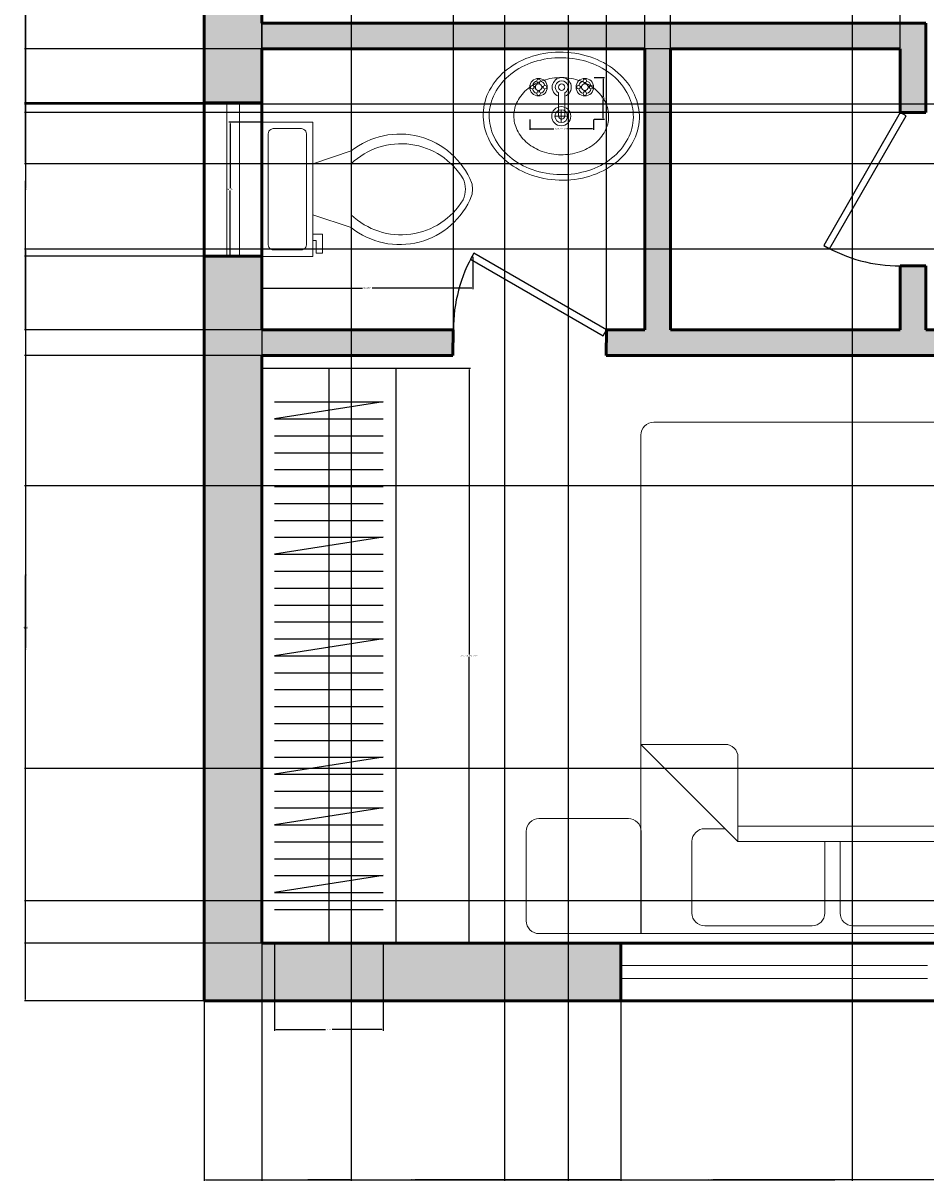
# Model space of a CAD drawing. Units: inches. Extents: x 1869 to 2483, y 2084 to 2479.
# Tile 1 of 7: x 1869 to 2010, y 2084 to 2265. Entities that reach past the tile are written whole.
import ezdxf

# ---------------------------------------------------------------- set-up
doc = ezdxf.new("R2010")
doc.units = ezdxf.units.IN
for name, color, linetype, lineweight in [('A-ANNO-DIMS', 2, 'Continuous', 18), ('A-DOOR', 3, 'Continuous', 25), ('A-FLOR-CASE', 9, 'Continuous', 25), ('A-FLOR-FIXT', 9, 'Continuous', 18), ('A-FURN', 8, 'Continuous', 18), ('A-GLAZ', 4, 'Continuous', 18), ('A-WALL', 7, 'Continuous', 50)]:
    doc.layers.add(name, color=color, linetype=linetype, lineweight=lineweight)
doc.layers.add('A-WALL-PATT', color=18, linetype='Continuous', lineweight=13, true_color=0x000000)
doc.styles.get("Standard").update_dxf_attribs({"font": 'arial.ttf'})
doc.dimstyles.get("Standard").update_dxf_attribs({"dimtxt": 0.18, "dimasz": 0.18, "dimexe": 0.18, "dimexo": 0.0625, "dimgap": 0.09, "dimtad": 0, "dimtih": 1, "dimtoh": 1, "dimdec": 4, "dimzin": 0, "dimdsep": 46, "dimtxsty": 'Standard', "dimcen": 0.09, "dimadec": 0, "dimazin": 0, "dimtfac": 1, "dimtdec": 4, "dimtofl": 0, "dimtmove": 0, "dimatfit": 3, "dimfxl": 1, "dimtolj": 1, "dimtzin": 0, "dimarcsym": 0})

# ---------------------------------------------------------------- blocks, each defined once
blk = doc.blocks.new('Sink - Oval top')
for p, q in [((-1, 0), (1, 0)), ((0, 1), (0, -1))]:
    blk.add_line(p, q)
for points in [[(-12.23, 0.39, 0.117634), (-11.46, -3.36, 0.104469), (-8.88, -6.8, 0.090016), (-5.08, -9.07, 0.08192), (-0.32, -10.02, 0.08192), (4.49, -9.38, 0.090016), (8.42, -7.36, 0.104469), (11.22, -4.09, 0.117634), (12.23, -0.39, 0.117634), (11.46, 3.36, 0.104469), (8.88, 6.8, 0.090016), (5.08, 9.07, 0.08192), (0.32, 10.02, 0.08192), (-4.49, 9.38, 0.090016), (-8.42, 7.36, 0.104469), (-11.22, 4.09, 0.117634)], [(-11.29, 0.16, 0.118622), (-10.52, -3.25, 0.104678), (-8.07, -6.36, 0.089562), (-4.54, -8.37, 0.081185), (-0.13, -9.15, 0.081185), (4.3, -8.49, 0.089562), (7.89, -6.58, 0.104678), (10.42, -3.55, 0.118622), (11.29, -0.16, 0.118622), (10.52, 3.25, 0.104678), (8.07, 6.36, 0.089562), (4.54, 8.37, 0.081185), (0.13, 9.15, 0.081185), (-4.3, 8.49, 0.089562), (-7.89, 6.58, 0.104678), (-10.42, 3.55, 0.118622)], [(-7.42, 0.08, 0.118283), (-6.91, -2.17, 0.104607), (-5.29, -4.21, 0.089718), (-2.97, -5.53, 0.081436), (-0.07, -6.04, 0.081436), (2.84, -5.59, 0.089718), (5.2, -4.33, 0.104607), (6.86, -2.32, 0.118283), (7.42, -0.08, 0.118283), (6.91, 2.17, 0.104607), (5.29, 4.21, 0.089718), (2.97, 5.53, 0.081436), (0.07, 6.04, 0.081436), (-2.84, 5.59, 0.089718), (-5.2, 4.33, 0.104607), (-6.86, 2.32, 0.118283)]]:
    blk.add_lwpolyline(points, format="xyb", close=True)
for radius in [1.5, 1]:
    blk.add_circle((0, 0), radius)
blk = doc.blocks.new('Faucet - Bathroom top')
for p, q in [((-4.107, 0.125), (-4.375, 0.125)), ((-3.75, 0.4788), (-3.75, 0.75)), ((-3.5, 0.482), (-3.5, 0.75)), ((-3.1461, 0.125), (-2.875, 0.125)), ((3.143, 0.125), (2.875, 0.125)), ((3.5, 0.4788), (3.5, 0.75)), ((3.75, 0.482), (3.75, 0.75)), ((4.1039, 0.125), (4.375, 0.125)), ((-4.1039, -0.125), (-4.375, -0.125)), ((-3.75, -0.4821), (-3.75, -0.75)), ((-3.5, -0.4789), (-3.5, -0.75)), ((-3.143, -0.125), (-2.875, -0.125)), ((-0.5, -0.8639), (-0.5, -4.5)), ((0.5, -4.5), (0.5, -0.8631)), ((3.1461, -0.125), (2.875, -0.125)), ((3.5, -0.4821), (3.5, -0.75)), ((3.75, -0.4789), (3.75, -0.75)), ((4.107, -0.125), (4.375, -0.125))]:
    blk.add_line(p, q)
for centre, radius in [((-3.625, 0), 1.375), ((-4.625, 0), 0.2795), ((-3.625, 0), 0.5), ((-3.625, 1), 0.2795), ((-2.625, 0), 0.2795), ((0, 0), 0.5), ((3.625, 0), 1.375), ((2.625, 0), 0.2795), ((3.625, 0), 0.5), ((3.625, 1), 0.2795), ((4.625, 0), 0.2795), ((-3.625, -1), 0.2795), ((3.625, -1), 0.2795)]:
    blk.add_circle(centre, radius)
for centre, radius, start, end in [((-3.625, 0), 1, 105.2407, 164.2093), ((-3.625, 0), 1, 16.44125, 74.07887), ((0, 0), 1.5, 289.6514, 250.3603), ((0, 0), 1, 300.3431, 239.7554), ((3.625, 0), 1, 106.12, 164.0884), ((3.625, 0), 1, 16.23422, 73.90469), ((-3.625, 0), 1, 196.2342, 253.9047), ((-3.625, 0), 1, 286.12, 344.0884), ((3.625, 0), 1, 196.4413, 254.0789), ((3.625, 0), 1, 285.2407, 344.2093), ((0, -4.5), 0.5, 180, 0)]:
    blk.add_arc(centre, radius, start, end)
blk = doc.blocks.new('Toilet - top')
for p, q in [((9.5, -6), (9.5, -2)), ((-10, -8.5), (-8, -8.5)), ((-10, -9.5), (-10, -8.5)), ((-8, -8.5), (-8, -8)), ((-7, -8), (-7, -9.5)), ((-4, -8), (-6, -14)), ((4, -8), (6, -14)), ((-7, -9.5), (-10, -9.5)), ((4, -14), (-4, -14))]:
    blk.add_line(p, q)
blk.add_lwpolyline([(10.5, -8), (10.5, 0), (-10.5, 0), (-10.5, -8)], close=True)
for points in [[(8.5, -1), (-8.5, -1)], [(-9.5, -2), (-9.5, -6)], [(-8.5, -7), (8.5, -7)]]:
    blk.add_lwpolyline(points)
for centre, radius, start, end in [((-8.62, -1.88), 0.884, 81.8699, 188.1301), ((8.62, -1.88), 0.884, 351.8699, 98.1301), ((-8.62, -6.12), 0.884, 171.8699, 278.1301), ((8.62, -6.12), 0.884, 261.8699, 8.1301), ((3.52, -21.58), 12.17, 141.4691, 247.9714), ((4.2, -21.82), 11.33, 136.3677, 238.9468), ((-3.52, -21.58), 12.17, 292.0284, 38.5307), ((-4.2, -21.82), 11.33, 301.053, 43.6321), ((0, -27.88), 4, 245.7318, 294.2682), ((0, -29), 4, 254.8605, 285.1395)]:
    blk.add_arc(centre, radius, start, end)
blk = doc.blocks.new('Bed - Queen')
for p, q in [((0, -78), (0, 0)), ((0, 0), (60, 0)), ((60, 0), (60, -78)), ((10, -1.2), (26.8, -1.2)), ((33.2, -1.2), (50, -1.2)), ((8, -14.4), (8, -3.2)), ((28.8, -3.2), (28.8, -14.4)), ((31.2, -14.4), (31.2, -3.2)), ((52, -3.2), (52, -14.4)), ((0, -14.4), (44.8, -14.4)), ((60, -29.6), (44.8, -14.4)), ((44.8, -14.4), (44.8, -27.6)), ((44.8, -16.8), (0, -16.8)), ((50, -16.4), (46.8, -16.4)), ((46.8, -29.6), (60, -29.6)), ((58, -80), (2, -80))]:
    blk.add_line(p, q)
for points in [[(0, 0), (-16, 0, 0.414214), (-18, -2), (-18, -16, 0.414214), (-16, -18), (-2, -18, 0.414214), (0, -16)], [(75.96, 0.02), (59.96, 0.02), (59.96, -15.98, 0.414214), (61.96, -17.98), (75.96, -17.98, 0.414214), (77.96, -15.98), (77.96, -1.98, 0.414214)]]:
    blk.add_lwpolyline(points, format="xyb", close=True)
for centre, start, end in [((10, -3.2), 90, 180), ((26.8, -3.2), 0, 90), ((33.2, -3.2), 90, 180), ((50, -3.2), 0, 90), ((50, -14.4), 270, 0), ((46.8, -27.6), 180, 270), ((2, -78), 180, 270), ((58, -78), 270, 0)]:
    blk.add_arc(centre, 2, start, end)
blk = doc.blocks.new('*U13')
for p, q in [((0, 0), (0, 6)), ((40, 0), (40, 6))]:
    blk.add_line(p, q)
blk.add_lwpolyline([(0, 0), (34.64, -20), (35.52, -18.48), (0.87, 1.52)], close=True)
blk.add_arc((0, 0), 40, 330, 0)
blk = doc.blocks.new('WIN-GLAZING-48IN')
for p, q in [((0, 2), (48, 2)), ((0, 0), (48, 0))]:
    blk.add_line(p, q)
blk = doc.blocks.new('WARDROBE-RAIL-90IN')
for p, q in [((8.5, 90), (8.5, 0)), ((0, 84.71), (17, 84.71)), ((17, 84.71), (0, 82.06)), ((0, 82.06), (17, 82.06)), ((0, 79.41), (17, 79.41)), ((0, 76.76), (17, 76.76)), ((0, 74.12), (17, 74.12)), ((0, 71.47), (17, 71.47)), ((0, 68.82), (17, 68.82)), ((0, 66.18), (17, 66.18)), ((0, 63.53), (17, 63.53)), ((17, 63.53), (0, 60.88)), ((0, 60.88), (17, 60.88)), ((0, 58.23), (17, 58.23)), ((0, 55.59), (17, 55.59)), ((0, 52.94), (17, 52.94)), ((0, 50.29), (17, 50.29)), ((0, 47.65), (17, 47.65)), ((17, 47.65), (0, 45)), ((0, 45), (17, 45)), ((0, 42.35), (17, 42.35)), ((0, 39.71), (17, 39.71)), ((0, 37.06), (17, 37.06)), ((0, 34.41), (17, 34.41)), ((0, 31.76), (17, 31.76)), ((0, 29.12), (17, 29.12)), ((17, 29.12), (0, 26.47)), ((0, 26.47), (17, 26.47)), ((0, 23.82), (17, 23.82)), ((0, 21.18), (17, 21.18)), ((17, 21.18), (0, 18.53)), ((0, 18.53), (17, 18.53)), ((0, 15.88), (17, 15.88)), ((0, 13.23), (17, 13.23)), ((0, 10.59), (17, 10.59)), ((17, 10.59), (0, 7.94)), ((0, 7.94), (17, 7.94)), ((0, 5.29), (17, 5.29))]:
    blk.add_line(p, q)
blk = doc.blocks.new('*D23')
at = {"layer": 'A-ANNO-DIMS', "color": 0, "lineweight": -2, "transparency": 16777216}
for p, q in [((1948.05, 2249.64), (1948.05, 2248.02)), ((1958.05, 2249.64), (1958.05, 2248.02)), ((1948.23, 2248.2), (1951.83, 2248.2)), ((1957.87, 2248.2), (1954.26, 2248.2))]:
    blk.add_line(p, q, dxfattribs=at)
at = {"layer": 'A-ANNO-DIMS', "color": 0, "transparency": 16777216}
for points in [[(1948.23, 2248.23), (1948.23, 2248.17), (1948.05, 2248.2)], [(1957.87, 2248.23), (1957.87, 2248.17), (1958.05, 2248.2)]]:
    blk.add_solid(points, dxfattribs=at)
at = {"layer": 'Defpoints', "color": 0, "transparency": 16777216}
for p in [(1948.05, 2249.7), (1958.05, 2249.7), (1958.05, 2248.2)]:
    blk.add_point(p, dxfattribs=at)
at = {"layer": 'A-ANNO-DIMS', "color": 0, "transparency": 16777216, "insert": (1953.05, 2248.2), "char_height": 0.18, "attachment_point": 5}
blk.add_mtext('\\A1;BASIN TAP 10 TYP.', dxfattribs=at)
blk = doc.blocks.new('*D24')
at = {"layer": 'A-ANNO-DIMS', "color": 0, "lineweight": -2, "transparency": 16777216}
for p, q in [((1958.11, 2256.2), (1959.73, 2256.2)), ((1959.55, 2256.02), (1959.55, 2253.13)), ((1959.55, 2249.88), (1959.55, 2252.77)), ((1958.11, 2249.7), (1959.73, 2249.7))]:
    blk.add_line(p, q, dxfattribs=at)
at = {"layer": 'A-ANNO-DIMS', "color": 0, "transparency": 16777216}
for points in [[(1959.52, 2256.02), (1959.58, 2256.02), (1959.55, 2256.2)], [(1959.52, 2249.88), (1959.58, 2249.88), (1959.55, 2249.7)]]:
    blk.add_solid(points, dxfattribs=at)
at = {"layer": 'Defpoints', "color": 0, "transparency": 16777216}
for p in [(1958.05, 2256.2), (1959.55, 2256.2), (1958.05, 2249.7)]:
    blk.add_point(p, dxfattribs=at)
at = {"layer": 'A-ANNO-DIMS', "color": 0, "transparency": 16777216, "insert": (1959.55, 2252.95), "char_height": 0.18, "attachment_point": 5}
blk.add_mtext('\\A1;7 TYP.', dxfattribs=at)
blk = doc.blocks.new('*D25')
at = {"layer": 'A-ANNO-DIMS', "color": 0, "lineweight": -2, "transparency": 16777216}
for p, q in [((1906.08, 2228.16), (1906.08, 2223.09)), ((1939.13, 2228.16), (1939.13, 2223.09)), ((1906.26, 2223.27), (1921.83, 2223.27)), ((1938.95, 2223.27), (1923.38, 2223.27))]:
    blk.add_line(p, q, dxfattribs=at)
at = {"layer": 'A-ANNO-DIMS', "color": 0, "transparency": 16777216}
for points in [[(1906.26, 2223.3), (1906.26, 2223.24), (1906.08, 2223.27)], [(1938.95, 2223.3), (1938.95, 2223.24), (1939.13, 2223.27)]]:
    blk.add_solid(points, dxfattribs=at)
at = {"layer": 'Defpoints', "color": 0, "transparency": 16777216}
for p in [(1906.08, 2228.22), (1939.13, 2228.22), (1906.08, 2223.27)]:
    blk.add_point(p, dxfattribs=at)
at = {"layer": 'A-ANNO-DIMS', "color": 0, "transparency": 16777216, "insert": (1922.6, 2223.27), "char_height": 0.18, "attachment_point": 5}
blk.add_mtext('\\A1;WC 33 TYP.', dxfattribs=at)
blk = doc.blocks.new('*D26')
at = {"layer": 'A-ANNO-DIMS', "color": 0, "lineweight": -2, "transparency": 16777216}
for p, q in [((1906.02, 2249.22), (1900.94, 2249.22)), ((1901.12, 2249.04), (1901.12, 2238.9)), ((1901.12, 2228.4), (1901.12, 2238.54)), ((1906.02, 2228.22), (1900.94, 2228.22))]:
    blk.add_line(p, q, dxfattribs=at)
at = {"layer": 'A-ANNO-DIMS', "color": 0, "transparency": 16777216}
for points in [[(1901.09, 2249.04), (1901.15, 2249.04), (1901.12, 2249.22)], [(1901.09, 2228.4), (1901.15, 2228.4), (1901.12, 2228.22)]]:
    blk.add_solid(points, dxfattribs=at)
at = {"layer": 'Defpoints', "color": 0, "transparency": 16777216}
for p in [(1901.12, 2249.22), (1906.08, 2249.22), (1906.08, 2228.22)]:
    blk.add_point(p, dxfattribs=at)
at = {"layer": 'A-ANNO-DIMS', "color": 0, "transparency": 16777216, "insert": (1901.12, 2238.72), "char_height": 0.18, "attachment_point": 5}
blk.add_mtext('\\A1;21 TYP.', dxfattribs=at)
blk = doc.blocks.new('*D27')
at = {"layer": 'A-ANNO-DIMS', "color": 0, "lineweight": -2, "transparency": 16777216}
for p, q in [((1925.14, 2210.72), (1938.76, 2210.72)), ((1938.58, 2210.54), (1938.58, 2165.91)), ((1938.58, 2120.9), (1938.58, 2165.54)), ((1925.14, 2120.72), (1938.76, 2120.72))]:
    blk.add_line(p, q, dxfattribs=at)
at = {"layer": 'A-ANNO-DIMS', "color": 0, "transparency": 16777216}
for points in [[(1938.55, 2210.54), (1938.61, 2210.54), (1938.58, 2210.72)], [(1938.55, 2120.9), (1938.61, 2120.9), (1938.58, 2120.72)]]:
    blk.add_solid(points, dxfattribs=at)
at = {"layer": 'Defpoints', "color": 0, "transparency": 16777216}
for p in [(1925.08, 2210.72), (1938.58, 2210.72), (1925.08, 2120.72)]:
    blk.add_point(p, dxfattribs=at)
at = {"layer": 'A-ANNO-DIMS', "color": 0, "transparency": 16777216, "insert": (1938.58, 2165.72), "char_height": 0.18, "attachment_point": 5}
blk.add_mtext('\\A1;WARDROBE RAIL 90 TYP.', dxfattribs=at)
blk = doc.blocks.new('*D28')
at = {"layer": 'A-ANNO-DIMS', "color": 0, "lineweight": -2, "transparency": 16777216}
for p, q in [((1908.08, 2120.66), (1908.08, 2107.04)), ((1925.08, 2120.66), (1925.08, 2107.04)), ((1908.26, 2107.22), (1916.06, 2107.22)), ((1924.9, 2107.22), (1917.1, 2107.22))]:
    blk.add_line(p, q, dxfattribs=at)
at = {"layer": 'A-ANNO-DIMS', "color": 0, "transparency": 16777216}
for points in [[(1908.26, 2107.25), (1908.26, 2107.19), (1908.08, 2107.22)], [(1924.9, 2107.25), (1924.9, 2107.19), (1925.08, 2107.22)]]:
    blk.add_solid(points, dxfattribs=at)
at = {"layer": 'Defpoints', "color": 0, "transparency": 16777216}
for p in [(1908.08, 2120.72), (1925.08, 2120.72), (1925.08, 2107.22)]:
    blk.add_point(p, dxfattribs=at)
at = {"layer": 'A-ANNO-DIMS', "color": 0, "transparency": 16777216, "insert": (1916.58, 2107.22), "char_height": 0.18, "attachment_point": 5}
blk.add_mtext('\\A1;17 TYP.', dxfattribs=at)
blk = doc.blocks.new('*D40')
at = {"layer": 'A-ANNO-DIMS', "color": 0, "lineweight": -2, "transparency": 16777216}
for p, q in [((1906.08, 2120.66), (1906.08, 2083.54)), ((2086.08, 2120.66), (2086.08, 2083.54)), ((1906.26, 2083.72), (1995.8, 2083.72)), ((2085.9, 2083.72), (1996.36, 2083.72))]:
    blk.add_line(p, q, dxfattribs=at)
at = {"layer": 'A-ANNO-DIMS', "color": 0, "transparency": 16777216}
for points in [[(1906.26, 2083.75), (1906.26, 2083.69), (1906.08, 2083.72)], [(2085.9, 2083.75), (2085.9, 2083.69), (2086.08, 2083.72)]]:
    blk.add_solid(points, dxfattribs=at)
at = {"layer": 'Defpoints', "color": 0, "transparency": 16777216}
for p in [(1906.08, 2120.72), (2086.08, 2120.72), (2086.08, 2083.72)]:
    blk.add_point(p, dxfattribs=at)
at = {"layer": 'A-ANNO-DIMS', "color": 0, "transparency": 16777216, "insert": (1996.08, 2083.72), "char_height": 0.18, "attachment_point": 5}
blk.add_mtext('\\A1;180', dxfattribs=at)
blk = doc.blocks.new('*D43')
at = {"layer": 'A-ANNO-DIMS', "color": 0, "lineweight": -2, "transparency": 16777216}
for p, q in [((1906.02, 2212.72), (1868.9, 2212.72)), ((1869.08, 2212.54), (1869.08, 2166.91)), ((1869.08, 2120.9), (1869.08, 2166.54)), ((1906.02, 2120.72), (1868.9, 2120.72))]:
    blk.add_line(p, q, dxfattribs=at)
at = {"layer": 'A-ANNO-DIMS', "color": 0, "transparency": 16777216}
for points in [[(1869.05, 2212.54), (1869.11, 2212.54), (1869.08, 2212.72)], [(1869.05, 2120.9), (1869.11, 2120.9), (1869.08, 2120.72)]]:
    blk.add_solid(points, dxfattribs=at)
at = {"layer": 'Defpoints', "color": 0, "transparency": 16777216}
for p in [(1869.08, 2212.72), (1906.08, 2212.72), (1906.08, 2120.72)]:
    blk.add_point(p, dxfattribs=at)
at = {"layer": 'A-ANNO-DIMS', "color": 0, "transparency": 16777216, "insert": (1869.08, 2166.72), "char_height": 0.18, "attachment_point": 5}
blk.add_mtext('\\A1;92', dxfattribs=at)
blk = doc.blocks.new('*D44')
at = {"layer": 'A-ANNO-DIMS', "color": 0, "lineweight": -2, "transparency": 16777216}
for p, q in [((1906.017379, 2260.72353), (1868.899879, 2260.72353)), ((1869.079879, 2260.54353), (1869.079879, 2238.90353)), ((1869.079879, 2216.90353), (1869.079879, 2238.54353)), ((1906.017379, 2216.72353), (1868.899879, 2216.72353))]:
    blk.add_line(p, q, dxfattribs=at)
at = {"layer": 'A-ANNO-DIMS', "color": 0, "transparency": 16777216}
for points in [[(1869.049879, 2260.54353), (1869.109879, 2260.54353), (1869.079879, 2260.72353)], [(1869.049879, 2216.90353), (1869.109879, 2216.90353), (1869.079879, 2216.72353)]]:
    blk.add_solid(points, dxfattribs=at)
at = {"layer": 'Defpoints', "color": 0, "transparency": 16777216}
for p in [(1869.079879, 2260.72353), (1906.079879, 2260.72353), (1906.079879, 2216.72353)]:
    blk.add_point(p, dxfattribs=at)
at = {"layer": 'A-ANNO-DIMS', "color": 0, "transparency": 16777216, "insert": (1869.079879, 2238.72353), "char_height": 0.18, "attachment_point": 5}
blk.add_mtext('\\A1;44', dxfattribs=at)
blk = doc.blocks.new('*D49')
at = {"layer": 'A-ANNO-DIMS', "color": 0, "lineweight": -2, "transparency": 16777216}
for p, q in [((1906.08, 2260.79), (1906.08, 2479.07)), ((1906.26, 2478.89), (1935.86, 2478.89)), ((1965.9, 2478.89), (1936.3, 2478.89)), ((1966.08, 2260.79), (1966.08, 2479.07))]:
    blk.add_line(p, q, dxfattribs=at)
at = {"layer": 'A-ANNO-DIMS', "color": 0, "transparency": 16777216}
for points in [[(1906.26, 2478.92), (1906.26, 2478.86), (1906.08, 2478.89)], [(1965.9, 2478.92), (1965.9, 2478.86), (1966.08, 2478.89)]]:
    blk.add_solid(points, dxfattribs=at)
at = {"layer": 'Defpoints', "color": 0, "transparency": 16777216}
for p in [(1966.08, 2478.89), (1906.08, 2260.72), (1966.08, 2260.72)]:
    blk.add_point(p, dxfattribs=at)
at = {"layer": 'A-ANNO-DIMS', "color": 0, "transparency": 16777216, "insert": (1936.08, 2478.89), "char_height": 0.18, "attachment_point": 5}
blk.add_mtext('\\A1;60', dxfattribs=at)
blk = doc.blocks.new('*D50')
at = {"layer": 'A-ANNO-DIMS', "color": 0, "lineweight": -2, "transparency": 16777216}
for p, q in [((1970.08, 2260.79), (1970.08, 2479.07)), ((1970.26, 2478.89), (1987.86, 2478.89)), ((2005.9, 2478.89), (1988.3, 2478.89)), ((2006.08, 2260.79), (2006.08, 2479.07))]:
    blk.add_line(p, q, dxfattribs=at)
at = {"layer": 'A-ANNO-DIMS', "color": 0, "transparency": 16777216}
for points in [[(1970.26, 2478.92), (1970.26, 2478.86), (1970.08, 2478.89)], [(2005.9, 2478.92), (2005.9, 2478.86), (2006.08, 2478.89)]]:
    blk.add_solid(points, dxfattribs=at)
at = {"layer": 'Defpoints', "color": 0, "transparency": 16777216}
for p in [(2006.08, 2478.89), (1970.08, 2260.72), (2006.08, 2260.72)]:
    blk.add_point(p, dxfattribs=at)
at = {"layer": 'A-ANNO-DIMS', "color": 0, "transparency": 16777216, "insert": (1988.08, 2478.89), "char_height": 0.18, "attachment_point": 5}
blk.add_mtext('\\A1;36', dxfattribs=at)
blk = doc.blocks.new('*D51')
at = {"layer": 'A-ANNO-DIMS', "color": 0, "lineweight": -2, "transparency": 16777216}
for p, q in [((1954.08, 2420.66), (1954.08, 2083.54)), ((1998.52, 2420.66), (1998.52, 2083.54)), ((1954.26, 2083.72), (1975.9, 2083.72)), ((1998.34, 2083.72), (1976.7, 2083.72))]:
    blk.add_line(p, q, dxfattribs=at)
at = {"layer": 'A-ANNO-DIMS', "color": 0, "transparency": 16777216}
for points in [[(1954.26, 2083.75), (1954.26, 2083.69), (1954.08, 2083.72)], [(1998.34, 2083.75), (1998.34, 2083.69), (1998.52, 2083.72)]]:
    blk.add_solid(points, dxfattribs=at)
at = {"layer": 'Defpoints', "color": 0, "transparency": 16777216}
for p in [(1954.08, 2420.72), (1998.52, 2420.72), (1998.52, 2083.72)]:
    blk.add_point(p, dxfattribs=at)
at = {"layer": 'A-ANNO-DIMS', "color": 0, "transparency": 16777216, "insert": (1976.3, 2083.72), "char_height": 0.18, "attachment_point": 5}
blk.add_mtext('\\A1;44.44', dxfattribs=at)
blk = doc.blocks.new('*D53')
at = {"layer": 'A-ANNO-DIMS', "color": 0, "lineweight": -2, "transparency": 16777216}
for p, q in [((1897.08, 2111.66), (1897.08, 2083.54)), ((1962.33, 2111.66), (1962.33, 2083.54)), ((1897.26, 2083.72), (1929.31, 2083.72)), ((1962.15, 2083.72), (1930.1, 2083.72))]:
    blk.add_line(p, q, dxfattribs=at)
at = {"layer": 'A-ANNO-DIMS', "color": 0, "transparency": 16777216}
for points in [[(1897.26, 2083.75), (1897.26, 2083.69), (1897.08, 2083.72)], [(1962.15, 2083.75), (1962.15, 2083.69), (1962.33, 2083.72)]]:
    blk.add_solid(points, dxfattribs=at)
at = {"layer": 'Defpoints', "color": 0, "transparency": 16777216}
for p in [(1897.08, 2111.72), (1962.33, 2111.72), (1962.33, 2083.72)]:
    blk.add_point(p, dxfattribs=at)
at = {"layer": 'A-ANNO-DIMS', "color": 0, "transparency": 16777216, "insert": (1929.71, 2083.72), "char_height": 0.18, "attachment_point": 5}
blk.add_mtext('\\A1;65.25', dxfattribs=at)
blk = doc.blocks.new('*D57')
at = {"layer": 'A-ANNO-DIMS', "color": 0, "lineweight": -2, "transparency": 16777216}
for p, q in [((2446.02, 2296.72), (1868.9, 2296.72)), ((1869.08, 2296.54), (1869.08, 2274.58)), ((1869.08, 2252.25), (1869.08, 2274.22)), ((2446.02, 2252.07), (1868.9, 2252.07))]:
    blk.add_line(p, q, dxfattribs=at)
at = {"layer": 'A-ANNO-DIMS', "color": 0, "transparency": 16777216}
for points in [[(1869.05, 2296.54), (1869.11, 2296.54), (1869.08, 2296.72)], [(1869.05, 2252.25), (1869.11, 2252.25), (1869.08, 2252.07)]]:
    blk.add_solid(points, dxfattribs=at)
at = {"layer": 'Defpoints', "color": 0, "transparency": 16777216}
for p in [(1869.08, 2296.72), (2446.08, 2296.72), (2446.08, 2252.07)]:
    blk.add_point(p, dxfattribs=at)
at = {"layer": 'A-ANNO-DIMS', "color": 0, "transparency": 16777216, "insert": (1869.08, 2274.4), "char_height": 0.18, "attachment_point": 5}
blk.add_mtext('\\A1;44.65', dxfattribs=at)
blk = doc.blocks.new('*D58')
at = {"layer": 'A-ANNO-DIMS', "color": 0, "lineweight": -2, "transparency": 16777216}
for p, q in [((1897.02, 2252.25), (1868.9, 2252.25)), ((1869.08, 2252.07), (1869.08, 2240.43)), ((1869.08, 2228.43), (1869.08, 2240.07)), ((1897.02, 2228.25), (1868.9, 2228.25))]:
    blk.add_line(p, q, dxfattribs=at)
at = {"layer": 'A-ANNO-DIMS', "color": 0, "transparency": 16777216}
for points in [[(1869.05, 2252.07), (1869.11, 2252.07), (1869.08, 2252.25)], [(1869.05, 2228.43), (1869.11, 2228.43), (1869.08, 2228.25)]]:
    blk.add_solid(points, dxfattribs=at)
at = {"layer": 'Defpoints', "color": 0, "transparency": 16777216}
for p in [(1869.08, 2252.25), (1897.08, 2252.25), (1897.08, 2228.25)]:
    blk.add_point(p, dxfattribs=at)
at = {"layer": 'A-ANNO-DIMS', "color": 0, "transparency": 16777216, "insert": (1869.08, 2240.25), "char_height": 0.18, "attachment_point": 5}
blk.add_mtext('\\A1;24', dxfattribs=at)
blk = doc.blocks.new('*D59')
at = {"layer": 'A-ANNO-DIMS', "color": 0, "lineweight": -2, "transparency": 16777216}
for p, q in [((1897.02, 2228.25), (1868.9, 2228.25)), ((1869.08, 2228.07), (1869.08, 2170.17)), ((1869.08, 2111.9), (1869.08, 2169.8)), ((1897.02, 2111.72), (1868.9, 2111.72))]:
    blk.add_line(p, q, dxfattribs=at)
at = {"layer": 'A-ANNO-DIMS', "color": 0, "transparency": 16777216}
for points in [[(1869.05, 2228.07), (1869.11, 2228.07), (1869.08, 2228.25)], [(1869.05, 2111.9), (1869.11, 2111.9), (1869.08, 2111.72)]]:
    blk.add_solid(points, dxfattribs=at)
at = {"layer": 'Defpoints', "color": 0, "transparency": 16777216}
for p in [(1869.08, 2228.25), (1897.08, 2228.25), (1897.08, 2111.72)]:
    blk.add_point(p, dxfattribs=at)
at = {"layer": 'A-ANNO-DIMS', "color": 0, "transparency": 16777216, "insert": (1869.08, 2169.99), "char_height": 0.18, "attachment_point": 5}
blk.add_mtext('\\A1;116.53', dxfattribs=at)
blk = doc.blocks.new('*D63')
at = {"layer": 'A-ANNO-DIMS', "color": 0, "lineweight": -2, "transparency": 16777216}
for p, q in [((2348.34, 2272.72), (1868.9, 2272.72)), ((1869.08, 2272.54), (1869.08, 2257.91)), ((1869.08, 2242.9), (1869.08, 2257.54)), ((2348.34, 2242.72), (1868.9, 2242.72))]:
    blk.add_line(p, q, dxfattribs=at)
at = {"layer": 'A-ANNO-DIMS', "color": 0, "transparency": 16777216}
for points in [[(1869.05, 2272.54), (1869.11, 2272.54), (1869.08, 2272.72)], [(1869.05, 2242.9), (1869.11, 2242.9), (1869.08, 2242.72)]]:
    blk.add_solid(points, dxfattribs=at)
at = {"layer": 'Defpoints', "color": 0, "transparency": 16777216}
for p in [(1869.08, 2272.72), (2348.4, 2272.72), (2348.4, 2242.72)]:
    blk.add_point(p, dxfattribs=at)
at = {"layer": 'A-ANNO-DIMS', "color": 0, "transparency": 16777216, "insert": (1869.08, 2257.72), "char_height": 0.18, "attachment_point": 5}
blk.add_mtext('\\A1;30', dxfattribs=at)
blk = doc.blocks.new('*D67')
at = {"layer": 'A-ANNO-DIMS', "color": 0, "lineweight": -2, "transparency": 16777216}
for p, q in [((1936.08, 2216.79), (1936.08, 2479.07)), ((1936.26, 2478.89), (1947.86, 2478.89)), ((1959.9, 2478.89), (1948.3, 2478.89)), ((1960.08, 2216.79), (1960.08, 2479.07))]:
    blk.add_line(p, q, dxfattribs=at)
at = {"layer": 'A-ANNO-DIMS', "color": 0, "transparency": 16777216}
for points in [[(1936.26, 2478.92), (1936.26, 2478.86), (1936.08, 2478.89)], [(1959.9, 2478.92), (1959.9, 2478.86), (1960.08, 2478.89)]]:
    blk.add_solid(points, dxfattribs=at)
at = {"layer": 'Defpoints', "color": 0, "transparency": 16777216}
for p in [(1960.08, 2478.89), (1936.08, 2216.72), (1960.08, 2216.72)]:
    blk.add_point(p, dxfattribs=at)
at = {"layer": 'A-ANNO-DIMS', "color": 0, "transparency": 16777216, "insert": (1948.08, 2478.89), "char_height": 0.18, "attachment_point": 5}
blk.add_mtext('\\A1;24', dxfattribs=at)
blk = doc.blocks.new('*D69')
at = {"layer": 'A-ANNO-DIMS', "color": 0, "lineweight": -2, "transparency": 16777216}
for p, q in [((1920.08, 2336.66), (1920.08, 2083.54)), ((1944.08, 2336.66), (1944.08, 2083.54)), ((1920.26, 2083.72), (1931.86, 2083.72)), ((1943.9, 2083.72), (1932.3, 2083.72))]:
    blk.add_line(p, q, dxfattribs=at)
at = {"layer": 'A-ANNO-DIMS', "color": 0, "transparency": 16777216}
for points in [[(1920.26, 2083.75), (1920.26, 2083.69), (1920.08, 2083.72)], [(1943.9, 2083.75), (1943.9, 2083.69), (1944.08, 2083.72)]]:
    blk.add_solid(points, dxfattribs=at)
at = {"layer": 'Defpoints', "color": 0, "transparency": 16777216}
for p in [(1920.08, 2336.72), (1944.08, 2336.72), (1944.08, 2083.72)]:
    blk.add_point(p, dxfattribs=at)
at = {"layer": 'A-ANNO-DIMS', "color": 0, "transparency": 16777216, "insert": (1932.08, 2083.72), "char_height": 0.18, "attachment_point": 5}
blk.add_mtext('\\A1;24', dxfattribs=at)
blk = doc.blocks.new('*D83')
at = {"layer": 'A-ANNO-DIMS', "color": 0, "lineweight": -2, "transparency": 16777216}
for p, q in [((1960.08, 2216.79), (1960.08, 2479.07)), ((1960.26, 2478.89), (1962.7, 2478.89)), ((1965.9, 2478.89), (1963.46, 2478.89)), ((1966.08, 2216.79), (1966.08, 2479.07))]:
    blk.add_line(p, q, dxfattribs=at)
at = {"layer": 'A-ANNO-DIMS', "color": 0, "transparency": 16777216}
for points in [[(1960.26, 2478.92), (1960.26, 2478.86), (1960.08, 2478.89)], [(1965.9, 2478.92), (1965.9, 2478.86), (1966.08, 2478.89)]]:
    blk.add_solid(points, dxfattribs=at)
at = {"layer": 'Defpoints', "color": 0, "transparency": 16777216}
for p in [(1966.08, 2478.89), (1960.08, 2216.72), (1966.08, 2216.72)]:
    blk.add_point(p, dxfattribs=at)
at = {"layer": 'A-ANNO-DIMS', "color": 0, "transparency": 16777216, "insert": (1963.08, 2478.89), "char_height": 0.18, "attachment_point": 5}
blk.add_mtext('\\A1;6.001', dxfattribs=at)
blk = doc.blocks.new('*D84')
at = {"layer": 'A-ANNO-DIMS', "color": 0, "lineweight": -2, "transparency": 16777216}
for p, q in [((1906.08, 2336.66), (1906.08, 2083.54)), ((1920.08, 2336.66), (1920.08, 2083.54)), ((1906.26, 2083.72), (1912.87, 2083.72)), ((1919.9, 2083.72), (1913.29, 2083.72))]:
    blk.add_line(p, q, dxfattribs=at)
at = {"layer": 'A-ANNO-DIMS', "color": 0, "transparency": 16777216}
for points in [[(1906.26, 2083.75), (1906.26, 2083.69), (1906.08, 2083.72)], [(1919.9, 2083.75), (1919.9, 2083.69), (1920.08, 2083.72)]]:
    blk.add_solid(points, dxfattribs=at)
at = {"layer": 'Defpoints', "color": 0, "transparency": 16777216}
for p in [(1906.08, 2336.72), (1920.08, 2336.72), (1920.08, 2083.72)]:
    blk.add_point(p, dxfattribs=at)
at = {"layer": 'A-ANNO-DIMS', "color": 0, "transparency": 16777216, "insert": (1913.08, 2083.72), "char_height": 0.18, "attachment_point": 5}
blk.add_mtext('\\A1;14', dxfattribs=at)
blk = doc.blocks.new('*D85')
at = {"layer": 'A-ANNO-DIMS', "color": 0, "lineweight": -2, "transparency": 16777216}
for p, q in [((2006.02, 2260.72), (1868.9, 2260.72)), ((1869.08, 2260.54), (1869.08, 2255.91)), ((1869.08, 2250.9), (1869.08, 2255.54)), ((2006.02, 2250.72), (1868.9, 2250.72))]:
    blk.add_line(p, q, dxfattribs=at)
at = {"layer": 'A-ANNO-DIMS', "color": 0, "transparency": 16777216}
for points in [[(1869.05, 2260.54), (1869.11, 2260.54), (1869.08, 2260.72)], [(1869.05, 2250.9), (1869.11, 2250.9), (1869.08, 2250.72)]]:
    blk.add_solid(points, dxfattribs=at)
at = {"layer": 'Defpoints', "color": 0, "transparency": 16777216}
for p in [(1869.08, 2260.72), (2006.08, 2260.72), (2006.08, 2250.72)]:
    blk.add_point(p, dxfattribs=at)
at = {"layer": 'A-ANNO-DIMS', "color": 0, "transparency": 16777216, "insert": (1869.08, 2255.72), "char_height": 0.18, "attachment_point": 5}
blk.add_mtext('\\A1;10', dxfattribs=at)
blk = doc.blocks.new('*D86')
at = {"layer": 'A-ANNO-DIMS', "color": 0, "lineweight": -2, "transparency": 16777216}
for p, q in [((2241.99, 2229.37), (1868.9, 2229.37)), ((1869.08, 2229.19), (1869.08, 2178.55)), ((1869.08, 2127.55), (1869.08, 2178.19)), ((2241.99, 2127.37), (1868.9, 2127.37))]:
    blk.add_line(p, q, dxfattribs=at)
at = {"layer": 'A-ANNO-DIMS', "color": 0, "transparency": 16777216}
for points in [[(1869.05, 2229.19), (1869.11, 2229.19), (1869.08, 2229.37)], [(1869.05, 2127.55), (1869.11, 2127.55), (1869.08, 2127.37)]]:
    blk.add_solid(points, dxfattribs=at)
at = {"layer": 'Defpoints', "color": 0, "transparency": 16777216}
for p in [(2242.05, 2229.37), (1869.08, 2127.37), (2242.05, 2127.37)]:
    blk.add_point(p, dxfattribs=at)
at = {"layer": 'A-ANNO-DIMS', "color": 0, "transparency": 16777216, "insert": (1869.08, 2178.37), "char_height": 0.18, "attachment_point": 5}
blk.add_mtext('\\A1;102', dxfattribs=at)
blk = doc.blocks.new('*D90')
at = {"layer": 'A-ANNO-DIMS', "color": 0, "lineweight": -2, "transparency": 16777216}
for p, q in [((2190.22, 2192.3), (1868.9, 2192.3)), ((1869.08, 2192.12), (1869.08, 2170.36)), ((1869.08, 2148.24), (1869.08, 2170)), ((2190.22, 2148.06), (1868.9, 2148.06))]:
    blk.add_line(p, q, dxfattribs=at)
at = {"layer": 'A-ANNO-DIMS', "color": 0, "transparency": 16777216}
for points in [[(1869.05, 2192.12), (1869.11, 2192.12), (1869.08, 2192.3)], [(1869.05, 2148.24), (1869.11, 2148.24), (1869.08, 2148.06)]]:
    blk.add_solid(points, dxfattribs=at)
at = {"layer": 'Defpoints', "color": 0, "transparency": 16777216}
for p in [(1869.08, 2192.3), (2190.29, 2192.3), (2190.29, 2148.06)]:
    blk.add_point(p, dxfattribs=at)
at = {"layer": 'A-ANNO-DIMS', "color": 0, "transparency": 16777216, "insert": (1869.08, 2170.18), "char_height": 0.18, "attachment_point": 5}
blk.add_mtext('\\A1;44.24', dxfattribs=at)

msp = doc.modelspace()

# ---------------------------------------------------------------- hatches: boundary and pattern name
at = {"layer": 'A-WALL-PATT'}
h = msp.add_hatch(color=256, dxfattribs=at)
h.dxf.hatch_style = 1
h.paths.add_polyline_path([(1998.5221, 2429.7235), (1897.0799, 2429.7235), (1897.0799, 2252.2488), (1906.0799, 2252.2488), (1906.0799, 2260.7235), (1966.0799, 2260.7235), (1966.0799, 2216.7235), (1960.0791, 2216.7235), (1960.0161, 2212.7235), (2050.0707, 2212.7235), (2050.1612, 2216.7235), (2010.0799, 2216.7235), (2010.0799, 2226.7235), (2006.0799, 2226.7235), (2006.0799, 2216.7235), (1970.0799, 2216.7235), (1970.0799, 2260.7235), (2006.0799, 2260.7235), (2006.0799, 2250.7235), (2010.0799, 2250.7235), (2010.0799, 2264.7235), (1906.0799, 2264.7235), (1906.0799, 2336.7235), (1920.0799, 2336.7235), (1920.0799, 2340.7235), (1906.0799, 2340.7235), (1906.0799, 2420.7235), (1950.0799, 2420.7235), (1950.0799, 2340.7235), (1944.0799, 2340.7235), (1944.0799, 2336.7235), (1950.0799, 2336.7235), (1950.0799, 2296.7235), (2050.0799, 2296.7235), (2050.0799, 2300.7235), (1954.0799, 2300.7235), (1954.0799, 2420.7235), (1998.5221, 2420.7235)])
h = msp.add_hatch(color=256, dxfattribs=at)
h.dxf.hatch_style = 1
h.paths.add_polyline_path([(1962.3331, 2120.7235), (1906.0799, 2120.7235), (1906.0799, 2210.7235), (1906.0799, 2212.7235), (1936.0131, 2212.7235), (1936.0762, 2216.7235), (1906.0799, 2216.7235), (1906.0799, 2228.2488), (1897.0799, 2228.2488), (1897.0799, 2111.7235), (1962.3331, 2111.7235)])

# ---------------------------------------------------------------- linework, layer by layer
at = {"layer": 'A-FLOR-CASE'}
for p, q in [((1906.0799, 2210.7235), (1927.0799, 2210.7235)), ((1927.0799, 2210.7235), (1927.0799, 2120.7235)), ((1927.0799, 2120.7235), (1906.0799, 2120.7235)), ((1906.0799, 2120.7235), (1927.0799, 2120.7235))]:
    msp.add_line(p, q, dxfattribs=at)
at = {"layer": 'A-GLAZ'}
for p, q in [((1900.5799, 2252.2488), (1900.5799, 2228.2488)), ((1902.5799, 2252.2488), (1902.5799, 2228.2488))]:
    msp.add_line(p, q, dxfattribs=at)
at = {"layer": 'A-WALL'}
for p, q in [((1906.0799, 2264.7235), (1906.0799, 2336.7235)), ((2010.0799, 2264.7235), (1906.0799, 2264.7235)), ((2010.0799, 2250.7235), (2010.0799, 2264.7235)), ((1906.0799, 2216.7235), (1906.0799, 2260.7235)), ((1966.0799, 2260.7235), (1906.0799, 2260.7235)), ((1966.0799, 2216.7235), (1966.0799, 2260.7235)), ((2006.0799, 2260.7235), (1970.0799, 2260.7235)), ((1970.0799, 2216.7235), (1970.0799, 2260.7235)), ((2006.0799, 2250.7235), (2006.0799, 2260.7235)), ((1897.0799, 2252.2488), (1906.0799, 2252.2488)), ((2006.0799, 2250.7235), (2010.0799, 2250.7235)), ((1906.0799, 2228.2488), (1897.0799, 2228.2488)), ((2006.0799, 2216.7235), (2006.0799, 2226.7235)), ((2006.0799, 2226.7235), (2010.0799, 2226.7235)), ((2010.0799, 2216.7235), (2010.0799, 2226.7235)), ((1936.0762, 2216.7235), (1906.0799, 2216.7235)), ((1936.0762, 2216.7235), (1936.0131, 2212.7235)), ((1960.0791, 2216.7235), (1960.0161, 2212.7235)), ((1966.0799, 2216.7235), (1960.0791, 2216.7235)), ((2006.0799, 2216.7235), (1970.0799, 2216.7235)), ((2050.1612, 2216.7235), (2010.0799, 2216.7235)), ((1906.0799, 2120.7235), (1906.0799, 2212.7235)), ((1936.0131, 2212.7235), (1906.0799, 2212.7235)), ((2050.0707, 2212.7235), (1960.0161, 2212.7235)), ((1906.0799, 2120.7235), (1906.0799, 2210.7235)), ((2086.0799, 2120.7235), (1906.0799, 2120.7235)), ((1962.3331, 2111.7235), (1962.3331, 2120.7235))]:
    msp.add_line(p, q, dxfattribs=at)
msp.add_lwpolyline([(2152.0799, 2111.7235), (1897.0799, 2111.7235), (1897.0799, 2429.7235), (2455.0799, 2429.7235), (2455.0799, 2111.7235), (2200.0799, 2111.7235)], dxfattribs=at)

# ---------------------------------------------------------------- block references
at = {"layer": 'A-DOOR', "xscale": 0.6, "yscale": 0.6, "zscale": 0.6}
for p, rotation in [((2006.0799, 2250.7235), 270), ((1960.0791, 2216.7235), 180)]:
    msp.add_blockref('*U13', p, dxfattribs=dict(at, rotation=rotation))
at = {"layer": 'A-FLOR-CASE'}
msp.add_blockref('WARDROBE-RAIL-90IN', (1908.08, 2120.724), dxfattribs=at)
at = {"layer": 'A-FLOR-FIXT'}
for name, p in [('Sink - Oval top', (1952.9805, 2250.1666)), ('Faucet - Bathroom top', (1953.0482, 2254.7034))]:
    msp.add_blockref(name, p, dxfattribs=at)
at = {"layer": 'A-FLOR-FIXT', "rotation": 90}
msp.add_blockref('Toilet - top', (1906.0799, 2238.7235), dxfattribs=at)
at = {"layer": 'A-FURN', "rotation": 180}
msp.add_blockref('Bed - Queen', (2025.4526, 2122.2569), dxfattribs=at)
at = {"layer": 'A-GLAZ'}
msp.add_blockref('WIN-GLAZING-48IN', (1962.333, 2115.224), dxfattribs=at)

# ---------------------------------------------------------------- dimensions: what is measured, and where the dimension line sits
at = {"layer": 'A-ANNO-DIMS'}
for base, p1, p2, override, picture, middle in [((1966.0799, 2478.8871), (1906.0799, 2260.7235), (1966.0799, 2260.7235), {"dimdec": 0, "dimlfac": 1, "dimrnd": 0, "dimzin": 0, "dimdsep": 46, "dimlunit": 2}, '*D49', (1936.0799, 2478.8871)), ((1960.0791, 2478.8871), (1936.0791, 2216.7235), (1960.0791, 2216.7235), {"dimdec": 0, "dimlfac": 1, "dimrnd": 0, "dimzin": 0, "dimdsep": 46, "dimlunit": 2}, '*D67', (1948.0791, 2478.8871)), ((1966.0799, 2478.8871), (1960.0791, 2216.7235), (1966.0799, 2216.7235), {"dimdec": 3, "dimlfac": 1, "dimrnd": 0, "dimzin": 0, "dimdsep": 46, "dimlunit": 2}, '*D83', (1963.0795, 2478.8871)), ((2006.0799, 2478.8871), (1970.0799, 2260.7235), (2006.0799, 2260.7235), {"dimdec": 0, "dimlfac": 1, "dimrnd": 0, "dimzin": 0, "dimdsep": 46, "dimlunit": 2}, '*D50', (1988.0799, 2478.8871)), ((1998.5221, 2083.7235), (1954.0799, 2420.7235), (1998.5221, 2420.7235), {"dimdec": 2, "dimlfac": 1, "dimrnd": 0, "dimzin": 0, "dimdsep": 46, "dimlunit": 2}, '*D51', (1976.301, 2083.7235)), ((1920.0799, 2083.7235), (1906.0799, 2336.7235), (1920.0799, 2336.7235), {"dimdec": 0, "dimlfac": 1, "dimrnd": 0, "dimzin": 0, "dimdsep": 46, "dimlunit": 2}, '*D84', (1913.0799, 2083.7235)), ((1944.0799, 2083.7235), (1920.0799, 2336.7235), (1944.0799, 2336.7235), {"dimdec": 0, "dimlfac": 1, "dimrnd": 0, "dimzin": 0, "dimdsep": 46, "dimlunit": 2}, '*D69', (1932.0799, 2083.7235)), ((2086.0799, 2083.7235), (1906.0799, 2120.7235), (2086.0799, 2120.7235), {"dimdec": 0, "dimlfac": 1, "dimrnd": 0, "dimzin": 0, "dimdsep": 46, "dimlunit": 2}, '*D40', (1996.0799, 2083.7235)), ((1962.3331, 2083.7235), (1897.0799, 2111.7235), (1962.3331, 2111.7235), {"dimdec": 2, "dimlfac": 1, "dimrnd": 0, "dimzin": 0, "dimdsep": 46, "dimlunit": 2}, '*D53', (1929.7065, 2083.7235))]:
    dim = msp.add_linear_dim(base=base, p1=p1, p2=p2, dimstyle='Standard', override=override, dxfattribs=at)
    dim.commit()
    dim.dimension.update_dxf_attribs({"geometry": picture, "text_midpoint": middle})
for base, p1, p2, override, picture, middle in [((1869.0799, 2296.7235), (2446.0799, 2252.0706), (2446.0799, 2296.7235), {"dimdec": 2, "dimlfac": 1, "dimrnd": 0, "dimzin": 0, "dimdsep": 46, "dimlunit": 2}, '*D57', (1869.0799, 2274.3971)), ((1869.0799, 2272.7235), (2348.3982, 2242.7235), (2348.3982, 2272.7235), {"dimdec": 0, "dimlfac": 1, "dimrnd": 0, "dimzin": 0, "dimdsep": 46, "dimlunit": 2}, '*D63', (1869.0799, 2257.7235)), ((1869.0799, 2260.7235), (1906.0799, 2216.7235), (1906.0799, 2260.7235), {"dimdec": 0, "dimlfac": 1, "dimrnd": 0, "dimzin": 0, "dimdsep": 46, "dimlunit": 2}, '*D44', (1869.0799, 2238.7235)), ((1869.0799, 2260.7235), (2006.0799, 2250.7235), (2006.0799, 2260.7235), {"dimdec": 0, "dimlfac": 1, "dimrnd": 0, "dimzin": 0, "dimdsep": 46, "dimlunit": 2}, '*D85', (1869.0799, 2255.7235)), ((1869.0799, 2252.2488), (1897.0799, 2228.2488), (1897.0799, 2252.2488), {"dimdec": 0, "dimlfac": 1, "dimrnd": 0, "dimzin": 0, "dimdsep": 46, "dimlunit": 2}, '*D58', (1869.0799, 2240.2488)), ((1869.0799, 2127.3727), (2242.0537, 2229.3727), (2242.0537, 2127.3727), {"dimdec": 0, "dimlfac": 1, "dimrnd": 0, "dimzin": 0, "dimdsep": 46, "dimlunit": 2}, '*D86', (1869.0799, 2178.3727)), ((1869.0799, 2228.2488), (1897.0799, 2111.7235), (1897.0799, 2228.2488), {"dimdec": 2, "dimlfac": 1, "dimrnd": 0, "dimzin": 0, "dimdsep": 46, "dimlunit": 2}, '*D59', (1869.0799, 2169.9862)), ((1869.0799, 2212.7235), (1906.0799, 2120.7235), (1906.0799, 2212.7235), {"dimdec": 0, "dimlfac": 1, "dimrnd": 0, "dimzin": 0, "dimdsep": 46, "dimlunit": 2}, '*D43', (1869.0799, 2166.7235)), ((1869.0799, 2192.3029), (2190.2869, 2148.0595), (2190.2869, 2192.3029), {"dimdec": 2, "dimlfac": 1, "dimrnd": 0, "dimzin": 0, "dimdsep": 46, "dimlunit": 2}, '*D90', (1869.0799, 2170.1812))]:
    dim = msp.add_linear_dim(base=base, p1=p1, p2=p2, angle=90, dimstyle='Standard', override=override, dxfattribs=at)
    dim.commit()
    dim.dimension.update_dxf_attribs({"geometry": picture, "text_midpoint": middle})
for base, p1, p2, angle, text, picture, middle in [((1959.54816, 2256.20344), (1958.04816, 2249.70336), (1958.04816, 2256.20344), 90, '<> TYP.', '*D24', (1959.54816, 2252.9534)), ((1901.1229, 2249.2235), (1906.0799, 2228.2235), (1906.0799, 2249.2235), 90, '<> TYP.', '*D26', (1901.1229, 2238.7235)), ((1906.0799, 2223.2666), (1939.1261, 2228.2235), (1906.0799, 2228.2235), 180, 'WC <> TYP.', '*D25', (1922.603, 2223.2666)), ((1938.5799, 2210.7235), (1925.0799, 2120.7235), (1925.0799, 2210.7235), 90, 'WARDROBE RAIL <> TYP.', '*D27', (1938.5799, 2165.7235))]:
    dim = msp.add_linear_dim(base=base, p1=p1, p2=p2, angle=angle, text=text, dimstyle='Standard', override={"dimdec": 0, "dimlfac": 1, "dimrnd": 0, "dimzin": 0, "dimdsep": 46, "dimlunit": 2}, dxfattribs=at)
    dim.commit()
    dim.dimension.update_dxf_attribs({"geometry": picture, "text_midpoint": middle})
for base, p1, p2, text, picture, middle in [((1958.0482, 2248.2034), (1948.0482, 2249.7034), (1958.0482, 2249.7034), 'BASIN TAP <> TYP.', '*D23', (1953.0482, 2248.2034)), ((1925.0799, 2107.2235), (1908.0799, 2120.7235), (1925.0799, 2120.7235), '<> TYP.', '*D28', (1916.5799, 2107.2235))]:
    dim = msp.add_linear_dim(base=base, p1=p1, p2=p2, text=text, dimstyle='Standard', override={"dimdec": 0, "dimlfac": 1, "dimrnd": 0, "dimzin": 0, "dimdsep": 46, "dimlunit": 2}, dxfattribs=at)
    dim.commit()
    dim.dimension.update_dxf_attribs({"geometry": picture, "text_midpoint": middle})

doc.saveas('drawing.dxf')
